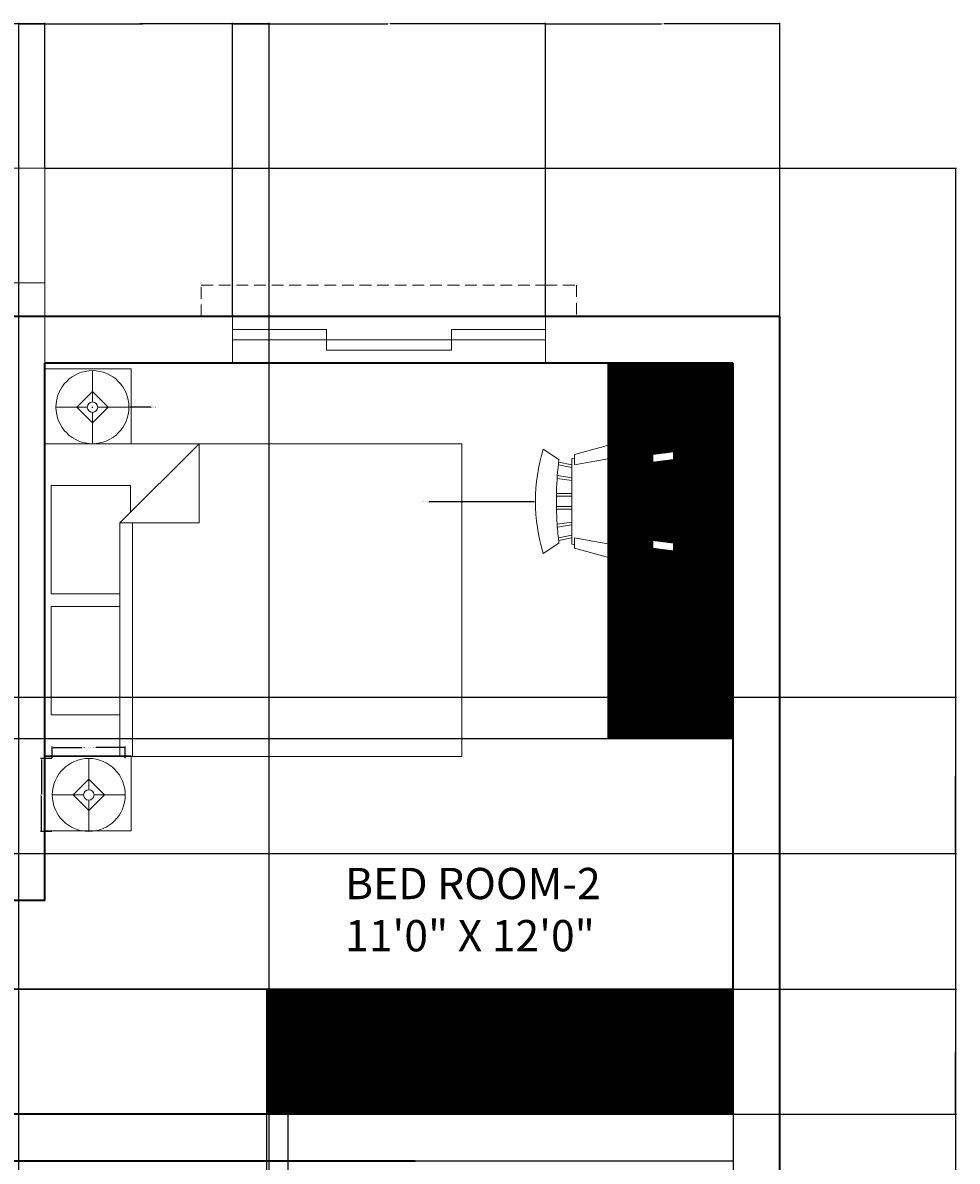
# Model space of a CAD drawing. Units: inches. Extents: x 6662 to 7211, y 5077 to 5683.
# Tile 9 of 9: x 7032 to 7211, y 5465 to 5683. Entities that reach past the tile are written whole.
import ezdxf

# ---------------------------------------------------------------- set-up
doc = ezdxf.new("R2010")
doc.units = ezdxf.units.IN
doc.header["$LTSCALE"] = 3
doc.header["$MEASUREMENT"] = 0
doc.linetypes.add('HIDDEN', pattern=[0.375, 0.25, -0.125])
for name, color, linetype, lineweight in [('A-ANNO-DIMS', 2, 'Continuous', 18), ('A-AREA-IDEN', 7, 'Continuous', 18), ('A-FLOR-CASE', 8, 'Continuous', 20), ('A-FLOR-CASE-PATT', 241, 'Continuous', 13), ('A-FLOR-PROJ', 7, 'Continuous', 18), ('A-FURN', 8, 'Continuous', 18), ('A-GLAZ', 4, 'Continuous', 18), ('A-GLAZ-OVHD', 4, 'HIDDEN', 13), ('A-WALL', 7, 'Continuous', 35)]:
    doc.layers.add(name, color=color, linetype=linetype, lineweight=lineweight)
doc.styles.get("Standard").update_dxf_attribs({"font": 'arial.ttf'})
doc.dimstyles.get("Standard").update_dxf_attribs({"dimtxt": 0.18, "dimasz": 0.18, "dimexe": 0.18, "dimexo": 0.0625, "dimgap": 0.09, "dimtad": 0, "dimtih": 1, "dimtoh": 1, "dimdec": 4, "dimzin": 0, "dimdsep": 46, "dimtxsty": 'Standard', "dimcen": 0.09, "dimadec": 0, "dimazin": 0, "dimtfac": 1, "dimtdec": 4, "dimtofl": 0, "dimtmove": 0, "dimatfit": 3, "dimfxl": 1, "dimtolj": 1, "dimtzin": 0, "dimarcsym": 0})

# ---------------------------------------------------------------- blocks, each defined once
blk = doc.blocks.new('Chair - Rocking')
for p, q in [((-8, -4.5), (-10, -1.5)), ((8, -4.5), (10, -1.5)), ((-4.5, -7), (-4.96674, -4.19951)), ((-4, -7), (-4.40532, -4.16272)), ((-1.5, -4.05012), (-1.5, -7)), ((-1, -7), (-1, -4.05012)), ((1, -7), (1, -4.04655)), ((1.5, -4.05012), (1.5, -7)), ((4, -7), (4.40187, -4.18694)), ((4.5, -7), (4.96761, -4.19437)), ((-7.5, -4.5), (-7, -7)), ((-6.5, -7), (-7.02225, -4.43)), ((6.5, -7), (7, -4.4057)), ((7.5, -4.5), (7, -7)), ((-9, -7.5), (-12, -18.49999)), ((-7, -7.5), (-9, -7.5)), ((-9, -18.49999), (-7, -7.5)), ((-8.23428, -6.99939), (-8.3093, -7.47958)), ((-8.23041, -7), (8.23915, -7)), ((7, -7.5), (9, -7.5)), ((9, -18.49999), (7, -7.5)), ((8.31071, -7.48854), (8.23449, -7.00073)), ((9, -7.5), (12, -18.49999)), ((-10.36644, -20.64523), (-10.5, -21.49999)), ((10.5, -21.49999), (10.3575, -20.58798)), ((-9, -22.49999), (-9.5, -26.49999)), ((0, -22.49999), (-9.5, -22.49999)), ((-8, -26.49999), (-7.5, -22.49999)), ((0, -22.49999), (9.5, -22.49999)), ((8, -26.49999), (7.5, -22.49999)), ((9, -22.49999), (9.5, -26.49999)), ((-9.5, -26.49999), (-8, -26.49999)), ((9.5, -26.49999), (8, -26.49999))]:
    blk.add_line(p, q)
for centre, radius, start, end in [((0, -34.08333), 34.08333, 72.93847, 107.0615), ((0, -68.25004), 64.25, 93.92211, 97.15267), ((0, -68.25004), 64.25, 82.84733, 93.92211), ((-10.5, -18.99999), 1.58114, 161.5651, 18.43495), ((10.5, -18.99999), 1.58114, 161.5651, 18.43495), ((-9.5, -21.49999), 1, 180, 270), ((9.5, -21.49999), 1, 270, 0)]:
    blk.add_arc(centre, radius, start, end)
blk = doc.blocks.new('Bed - Queen')
for p, q in [((0, -80.00003), (0, 0)), ((0, 0), (59.99999, 0)), ((59.99999, 0), (59.99999, -80.00003)), ((7.99999, -1.2), (28.79998, -1.2)), ((7.99999, -14.4), (7.99999, -1.2)), ((28.79998, -1.2), (28.79998, -14.4)), ((31.19999, -1.2), (51.99999, -1.2)), ((31.19999, -14.4), (31.19999, -1.2)), ((51.99999, -1.2), (51.99999, -16.4)), ((0, -14.4), (44.8, -14.4)), ((59.99999, -29.6), (44.8, -14.4)), ((44.8, -14.4), (44.8, -29.6)), ((44.8, -16.8), (0, -16.8)), ((51.99999, -16.4), (46.79936, -16.4)), ((44.8, -29.6), (59.99999, -29.6)), ((59.99999, -80.00003), (0, -80.00003))]:
    blk.add_line(p, q)
blk = doc.blocks.new('Lamp - Table')
for p, q in [((0, 7), (0, 1)), ((0, 3), (-3, 0)), ((3, 0), (0, 3)), ((-1, 0), (-7, 0)), ((-3, 0), (0, -3)), ((0, -3), (3, 0)), ((1, 0), (7, 0)), ((0, -1), (0, -7))]:
    blk.add_line(p, q)
for radius in [7, 1]:
    blk.add_circle((0, 0), radius)
blk = doc.blocks.new('BEDSIDE-TABLE')
blk.add_lwpolyline([(0, 14.35), (16.56, 14.35), (16.56, 0), (0, 0)], close=True)
blk = doc.blocks.new('*D16')
at = {"layer": 'A-ANNO-DIMS', "color": 0, "lineweight": -2, "ltscale": 3, "transparency": 16777216}
for p, q in [((7037.28, 5541.89), (7037.28, 5544.11)), ((7037.46, 5543.93), (7042.94, 5543.93)), ((7051.1, 5543.93), (7045.62, 5543.93)), ((7051.28, 5541.89), (7051.28, 5544.11))]:
    blk.add_line(p, q, dxfattribs=at)
at = {"layer": 'A-ANNO-DIMS', "color": 0, "ltscale": 3, "transparency": 16777216}
for points in [[(7037.46, 5543.96), (7037.46, 5543.9), (7037.28, 5543.93)], [(7051.1, 5543.96), (7051.1, 5543.9), (7051.28, 5543.93)]]:
    blk.add_solid(points, dxfattribs=at)
at = {"layer": 'Defpoints', "color": 0, "ltscale": 3, "transparency": 16777216}
for p in [(7051.28, 5543.93), (7037.28, 5541.83), (7051.28, 5541.83)]:
    blk.add_point(p, dxfattribs=at)
at = {"layer": 'A-ANNO-DIMS', "color": 0, "ltscale": 3, "transparency": 16777216, "insert": (7044.28, 5543.93), "char_height": 0.18, "attachment_point": 5}
blk.add_mtext('\\A1;TABLE LAMP 14 TYP.', dxfattribs=at)
blk = doc.blocks.new('*D17')
at = {"layer": 'A-ANNO-DIMS', "color": 0, "lineweight": -2, "ltscale": 3, "transparency": 16777216}
for p, q in [((7037.21, 5541.83), (7035, 5541.83)), ((7035.18, 5541.65), (7035.18, 5535.01)), ((7035.18, 5528.01), (7035.18, 5534.65)), ((7037.21, 5527.83), (7035, 5527.83))]:
    blk.add_line(p, q, dxfattribs=at)
at = {"layer": 'A-ANNO-DIMS', "color": 0, "ltscale": 3, "transparency": 16777216}
for points in [[(7035.15, 5541.65), (7035.21, 5541.65), (7035.18, 5541.83)], [(7035.15, 5528.01), (7035.21, 5528.01), (7035.18, 5527.83)]]:
    blk.add_solid(points, dxfattribs=at)
at = {"layer": 'Defpoints', "color": 0, "ltscale": 3, "transparency": 16777216}
for p in [(7035.18, 5541.83), (7037.28, 5541.83), (7037.28, 5527.83)]:
    blk.add_point(p, dxfattribs=at)
at = {"layer": 'A-ANNO-DIMS', "color": 0, "ltscale": 3, "transparency": 16777216, "insert": (7035.18, 5534.83), "char_height": 0.18, "attachment_point": 5}
blk.add_mtext('\\A1;14 TYP.', dxfattribs=at)
blk = doc.blocks.new('*D41')
at = {"layer": 'A-ANNO-DIMS', "color": 0, "lineweight": -2, "ltscale": 3, "transparency": 16777216}
for p, q in [((7035.92, 5655.02), (7210.74, 5655.02)), ((7210.56, 5654.84), (7210.56, 5379.99)), ((7210.56, 5104.78), (7210.56, 5379.63)), ((7010.92, 5104.6), (7210.74, 5104.6))]:
    blk.add_line(p, q, dxfattribs=at)
at = {"layer": 'A-ANNO-DIMS', "color": 0, "ltscale": 3, "transparency": 16777216}
for points in [[(7210.53, 5654.84), (7210.59, 5654.84), (7210.56, 5655.02)], [(7210.53, 5104.78), (7210.59, 5104.78), (7210.56, 5104.6)]]:
    blk.add_solid(points, dxfattribs=at)
at = {"layer": 'Defpoints', "color": 0, "ltscale": 3, "transparency": 16777216}
for p in [(7035.86, 5655.02), (7210.56, 5655.02), (7010.86, 5104.6)]:
    blk.add_point(p, dxfattribs=at)
at = {"layer": 'A-ANNO-DIMS', "color": 0, "ltscale": 3, "transparency": 16777216, "insert": (7210.56, 5379.81), "char_height": 0.18, "attachment_point": 5}
blk.add_mtext('\\A1;550.4', dxfattribs=at)
blk = doc.blocks.new('*D46')
at = {"layer": 'A-ANNO-DIMS', "color": 0, "lineweight": -2, "ltscale": 3, "transparency": 16777216}
for p, q in [((6869.86, 5655.08), (6869.86, 5682.9)), ((6870.04, 5682.72), (6952.58, 5682.72)), ((7035.68, 5682.72), (6953.14, 5682.72)), ((7035.86, 5655.08), (7035.86, 5682.9))]:
    blk.add_line(p, q, dxfattribs=at)
at = {"layer": 'A-ANNO-DIMS', "color": 0, "ltscale": 3, "transparency": 16777216}
for points in [[(6870.04, 5682.75), (6870.04, 5682.69), (6869.86, 5682.72)], [(7035.68, 5682.75), (7035.68, 5682.69), (7035.86, 5682.72)]]:
    blk.add_solid(points, dxfattribs=at)
at = {"layer": 'Defpoints', "color": 0, "ltscale": 3, "transparency": 16777216}
for p in [(7035.86, 5682.72), (6869.86, 5655.02), (7035.86, 5655.02)]:
    blk.add_point(p, dxfattribs=at)
at = {"layer": 'A-ANNO-DIMS', "color": 0, "ltscale": 3, "transparency": 16777216, "insert": (6952.86, 5682.72), "char_height": 0.18, "attachment_point": 5}
blk.add_mtext('\\A1;166', dxfattribs=at)
blk = doc.blocks.new('*D47')
at = {"layer": 'A-ANNO-DIMS', "color": 0, "lineweight": -2, "ltscale": 3, "transparency": 16777216}
for p, q in [((7035.86, 5655.08), (7035.86, 5682.9)), ((7036.04, 5682.72), (7053.64, 5682.72)), ((7071.68, 5682.72), (7054.08, 5682.72)), ((7071.86, 5626.66), (7071.86, 5682.9))]:
    blk.add_line(p, q, dxfattribs=at)
at = {"layer": 'A-ANNO-DIMS', "color": 0, "ltscale": 3, "transparency": 16777216}
for points in [[(7036.04, 5682.75), (7036.04, 5682.69), (7035.86, 5682.72)], [(7071.68, 5682.75), (7071.68, 5682.69), (7071.86, 5682.72)]]:
    blk.add_solid(points, dxfattribs=at)
at = {"layer": 'Defpoints', "color": 0, "ltscale": 3, "transparency": 16777216}
for p in [(7071.86, 5682.72), (7035.86, 5655.02), (7071.86, 5626.6)]:
    blk.add_point(p, dxfattribs=at)
at = {"layer": 'A-ANNO-DIMS', "color": 0, "ltscale": 3, "transparency": 16777216, "insert": (7053.86, 5682.72), "char_height": 0.18, "attachment_point": 5}
blk.add_mtext('\\A1;36', dxfattribs=at)
blk = doc.blocks.new('*D48')
at = {"layer": 'A-ANNO-DIMS', "color": 0, "lineweight": -2, "ltscale": 3, "transparency": 16777216}
for p, q in [((7071.86, 5626.66), (7071.86, 5682.9)), ((7072.04, 5682.72), (7101.64, 5682.72)), ((7131.68, 5682.72), (7102.08, 5682.72)), ((7131.86, 5626.66), (7131.86, 5682.9))]:
    blk.add_line(p, q, dxfattribs=at)
at = {"layer": 'A-ANNO-DIMS', "color": 0, "ltscale": 3, "transparency": 16777216}
for points in [[(7072.04, 5682.75), (7072.04, 5682.69), (7071.86, 5682.72)], [(7131.68, 5682.75), (7131.68, 5682.69), (7131.86, 5682.72)]]:
    blk.add_solid(points, dxfattribs=at)
at = {"layer": 'Defpoints', "color": 0, "ltscale": 3, "transparency": 16777216}
for p in [(7131.86, 5682.72), (7071.86, 5626.6), (7131.86, 5626.6)]:
    blk.add_point(p, dxfattribs=at)
at = {"layer": 'A-ANNO-DIMS', "color": 0, "ltscale": 3, "transparency": 16777216, "insert": (7101.86, 5682.72), "char_height": 0.18, "attachment_point": 5}
blk.add_mtext('\\A1;60', dxfattribs=at)
blk = doc.blocks.new('*D49')
at = {"layer": 'A-ANNO-DIMS', "color": 0, "lineweight": -2, "ltscale": 3, "transparency": 16777216}
for p, q in [((7131.86, 5626.66), (7131.86, 5682.9)), ((7132.04, 5682.72), (7154.13, 5682.72)), ((7176.68, 5682.72), (7154.58, 5682.72)), ((7176.86, 5626.66), (7176.86, 5682.9))]:
    blk.add_line(p, q, dxfattribs=at)
at = {"layer": 'A-ANNO-DIMS', "color": 0, "ltscale": 3, "transparency": 16777216}
for points in [[(7132.04, 5682.75), (7132.04, 5682.69), (7131.86, 5682.72)], [(7176.68, 5682.75), (7176.68, 5682.69), (7176.86, 5682.72)]]:
    blk.add_solid(points, dxfattribs=at)
at = {"layer": 'Defpoints', "color": 0, "ltscale": 3, "transparency": 16777216}
for p in [(7176.86, 5682.72), (7131.86, 5626.6), (7176.86, 5626.6)]:
    blk.add_point(p, dxfattribs=at)
at = {"layer": 'A-ANNO-DIMS', "color": 0, "ltscale": 3, "transparency": 16777216, "insert": (7154.36, 5682.72), "char_height": 0.18, "attachment_point": 5}
blk.add_mtext('\\A1;45', dxfattribs=at)
blk = doc.blocks.new('*D68')
at = {"layer": 'A-ANNO-DIMS', "color": 0, "lineweight": -2, "ltscale": 3, "transparency": 16777216}
for p, q in [((6878.92, 5553.6), (7210.74, 5553.6)), ((7210.56, 5553.42), (7210.56, 5538.78)), ((7210.56, 5523.78), (7210.56, 5538.42)), ((6878.92, 5523.6), (7210.74, 5523.6))]:
    blk.add_line(p, q, dxfattribs=at)
at = {"layer": 'A-ANNO-DIMS', "color": 0, "ltscale": 3, "transparency": 16777216}
for points in [[(7210.53, 5553.42), (7210.59, 5553.42), (7210.56, 5553.6)], [(7210.53, 5523.78), (7210.59, 5523.78), (7210.56, 5523.6)]]:
    blk.add_solid(points, dxfattribs=at)
at = {"layer": 'Defpoints', "color": 0, "ltscale": 3, "transparency": 16777216}
for p in [(6878.86, 5553.6), (7210.56, 5553.6), (6878.86, 5523.6)]:
    blk.add_point(p, dxfattribs=at)
at = {"layer": 'A-ANNO-DIMS', "color": 0, "ltscale": 3, "transparency": 16777216, "insert": (7210.56, 5538.6), "char_height": 0.18, "attachment_point": 5}
blk.add_mtext('\\A1;30', dxfattribs=at)
blk = doc.blocks.new('*D75')
at = {"layer": 'A-ANNO-DIMS', "color": 0, "lineweight": -2, "ltscale": 3, "transparency": 16777216}
for p, q in [((7030.86, 5179.16), (7030.86, 5682.9)), ((7031.04, 5682.72), (7054.64, 5682.72)), ((7078.68, 5682.72), (7055.08, 5682.72)), ((7078.86, 5179.16), (7078.86, 5682.9))]:
    blk.add_line(p, q, dxfattribs=at)
at = {"layer": 'A-ANNO-DIMS', "color": 0, "ltscale": 3, "transparency": 16777216}
for points in [[(7031.04, 5682.75), (7031.04, 5682.69), (7030.86, 5682.72)], [(7078.68, 5682.75), (7078.68, 5682.69), (7078.86, 5682.72)]]:
    blk.add_solid(points, dxfattribs=at)
at = {"layer": 'Defpoints', "color": 0, "ltscale": 3, "transparency": 16777216}
for p in [(7078.86, 5682.72), (7030.86, 5179.1), (7078.86, 5179.1)]:
    blk.add_point(p, dxfattribs=at)
at = {"layer": 'A-ANNO-DIMS', "color": 0, "ltscale": 3, "transparency": 16777216, "insert": (7054.86, 5682.72), "char_height": 0.18, "attachment_point": 5}
blk.add_mtext('\\A1;48', dxfattribs=at)
blk = doc.blocks.new('*D76')
at = {"layer": 'A-ANNO-DIMS', "color": 0, "lineweight": -2, "ltscale": 3, "transparency": 16777216}
for p, q in [((7167.8, 5464.6), (6661.98, 5464.6)), ((6662.16, 5464.42), (6662.16, 5449.65)), ((6662.16, 5434.53), (6662.16, 5449.29)), ((7167.8, 5434.35), (6661.98, 5434.35))]:
    blk.add_line(p, q, dxfattribs=at)
at = {"layer": 'A-ANNO-DIMS', "color": 0, "ltscale": 3, "transparency": 16777216}
for points in [[(6662.13, 5464.42), (6662.19, 5464.42), (6662.16, 5464.6)], [(6662.13, 5434.53), (6662.19, 5434.53), (6662.16, 5434.35)]]:
    blk.add_solid(points, dxfattribs=at)
at = {"layer": 'Defpoints', "color": 0, "ltscale": 3, "transparency": 16777216}
for p in [(7167.86, 5464.6), (6662.16, 5434.35), (7167.86, 5434.35)]:
    blk.add_point(p, dxfattribs=at)
at = {"layer": 'A-ANNO-DIMS', "color": 0, "ltscale": 3, "transparency": 16777216, "insert": (6662.16, 5449.47), "char_height": 0.18, "attachment_point": 5}
blk.add_mtext('\\A1;30.25', dxfattribs=at)
blk = doc.blocks.new('*D80')
at = {"layer": 'A-ANNO-DIMS', "color": 0, "lineweight": -2, "ltscale": 3, "transparency": 16777216}
for p, q in [((6825.96, 5497.6), (7210.74, 5497.6)), ((7210.56, 5497.42), (7210.56, 5485.78)), ((7210.56, 5473.78), (7210.56, 5485.42)), ((6825.96, 5473.6), (7210.74, 5473.6))]:
    blk.add_line(p, q, dxfattribs=at)
at = {"layer": 'A-ANNO-DIMS', "color": 0, "ltscale": 3, "transparency": 16777216}
for points in [[(7210.53, 5497.42), (7210.59, 5497.42), (7210.56, 5497.6)], [(7210.53, 5473.78), (7210.59, 5473.78), (7210.56, 5473.6)]]:
    blk.add_solid(points, dxfattribs=at)
at = {"layer": 'Defpoints', "color": 0, "ltscale": 3, "transparency": 16777216}
for p in [(6825.9, 5497.6), (7210.56, 5497.6), (6825.9, 5473.6)]:
    blk.add_point(p, dxfattribs=at)
at = {"layer": 'A-ANNO-DIMS', "color": 0, "ltscale": 3, "transparency": 16777216, "insert": (7210.56, 5485.6), "char_height": 0.18, "attachment_point": 5}
blk.add_mtext('\\A1;24', dxfattribs=at)
blk = doc.blocks.new('*D81')
at = {"layer": 'A-ANNO-DIMS', "color": 0, "lineweight": -2, "ltscale": 3, "transparency": 16777216}
for p, q in [((7078.36, 5473.54), (7078.36, 5076.72)), ((7167.86, 5473.54), (7167.86, 5076.72)), ((7078.54, 5076.9), (7122.78, 5076.9)), ((7167.68, 5076.9), (7123.43, 5076.9))]:
    blk.add_line(p, q, dxfattribs=at)
at = {"layer": 'A-ANNO-DIMS', "color": 0, "ltscale": 3, "transparency": 16777216}
for points in [[(7078.54, 5076.93), (7078.54, 5076.87), (7078.36, 5076.9)], [(7167.68, 5076.93), (7167.68, 5076.87), (7167.86, 5076.9)]]:
    blk.add_solid(points, dxfattribs=at)
at = {"layer": 'Defpoints', "color": 0, "ltscale": 3, "transparency": 16777216}
for p in [(7078.36, 5473.6), (7167.86, 5473.6), (7167.86, 5076.9)]:
    blk.add_point(p, dxfattribs=at)
at = {"layer": 'A-ANNO-DIMS', "color": 0, "ltscale": 3, "transparency": 16777216, "insert": (7123.11, 5076.9), "char_height": 0.18, "attachment_point": 5}
blk.add_mtext('\\A1;89.5', dxfattribs=at)
blk = doc.blocks.new('*D82')
at = {"layer": 'A-ANNO-DIMS', "color": 0, "lineweight": -2, "ltscale": 3, "transparency": 16777216}
for p, q in [((7167.8, 5545.6), (6661.98, 5545.6)), ((6662.16, 5545.42), (6662.16, 5521.78)), ((6662.16, 5497.78), (6662.16, 5521.42)), ((7167.8, 5497.6), (6661.98, 5497.6))]:
    blk.add_line(p, q, dxfattribs=at)
at = {"layer": 'A-ANNO-DIMS', "color": 0, "ltscale": 3, "transparency": 16777216}
for points in [[(6662.13, 5545.42), (6662.19, 5545.42), (6662.16, 5545.6)], [(6662.13, 5497.78), (6662.19, 5497.78), (6662.16, 5497.6)]]:
    blk.add_solid(points, dxfattribs=at)
at = {"layer": 'Defpoints', "color": 0, "ltscale": 3, "transparency": 16777216}
for p in [(6662.16, 5545.6), (7167.86, 5545.6), (7167.86, 5497.6)]:
    blk.add_point(p, dxfattribs=at)
at = {"layer": 'A-ANNO-DIMS', "color": 0, "ltscale": 3, "transparency": 16777216, "insert": (6662.16, 5521.6), "char_height": 0.18, "attachment_point": 5}
blk.add_mtext('\\A1;48', dxfattribs=at)
blk = doc.blocks.new('*D103')
at = {"layer": 'A-ANNO-DIMS', "color": 0, "lineweight": -2, "ltscale": 3, "transparency": 16777216}
for p, q in [((7082.65, 5477.61), (7082.47, 5477.61)), ((7082.47, 5477.61), (7082.47, 5441.64)), ((7082.38, 5381.21), (7082.56, 5381.21)), ((7082.47, 5381.12), (7082.47, 5381.3))]:
    blk.add_line(p, q, dxfattribs=at)
at = {"layer": 'A-ANNO-DIMS', "color": 0, "ltscale": 3, "transparency": 16777216}
blk.add_solid([(7082.44, 5441.64), (7082.5, 5441.64), (7082.47, 5441.46)], dxfattribs=at)
at = {"layer": 'Defpoints', "color": 0, "ltscale": 3, "transparency": 16777216}
for p in [(7082.47, 5441.46), (7082.47, 5381.21)]:
    blk.add_point(p, dxfattribs=at)
at = {"layer": 'A-ANNO-DIMS', "color": 0, "ltscale": 3, "transparency": 16777216, "insert": (7083.32, 5477.61), "char_height": 0.18, "attachment_point": 5}
blk.add_mtext('\\A1;2X R60.25', dxfattribs=at)
blk = doc.blocks.new('*D105')
at = {"layer": 'A-ANNO-DIMS', "color": 0, "lineweight": -2, "ltscale": 3, "transparency": 16777216}
for p, q in [((7109.51, 5591.13), (7129.78, 5591.13)), ((7163.96, 5591.13), (7164.14, 5591.13)), ((7164.05, 5591.04), (7164.05, 5591.22))]:
    blk.add_line(p, q, dxfattribs=at)
at = {"layer": 'A-ANNO-DIMS', "color": 0, "ltscale": 3, "transparency": 16777216}
blk.add_solid([(7129.78, 5591.16), (7129.78, 5591.1), (7129.96, 5591.13)], dxfattribs=at)
at = {"layer": 'Defpoints', "color": 0, "ltscale": 3, "transparency": 16777216}
for p in [(7129.96, 5591.13), (7164.05, 5591.13)]:
    blk.add_point(p, dxfattribs=at)
at = {"layer": 'A-ANNO-DIMS', "color": 0, "ltscale": 3, "transparency": 16777216, "insert": (7108.84, 5591.13), "char_height": 0.18, "attachment_point": 5}
blk.add_mtext('\\A1;3X R34.08', dxfattribs=at)
blk = doc.blocks.new('*D106')
at = {"layer": 'A-ANNO-DIMS', "color": 0, "lineweight": -2, "ltscale": 3, "transparency": 16777216}
for p, q in [((7044.89, 5609.19), (7045.07, 5609.19)), ((7044.98, 5609.1), (7044.98, 5609.28)), ((7056.18, 5609.19), (7052.16, 5609.19))]:
    blk.add_line(p, q, dxfattribs=at)
at = {"layer": 'A-ANNO-DIMS', "color": 0, "ltscale": 3, "transparency": 16777216}
blk.add_solid([(7052.16, 5609.22), (7052.16, 5609.16), (7051.98, 5609.19)], dxfattribs=at)
at = {"layer": 'Defpoints', "color": 0, "ltscale": 3, "transparency": 16777216}
for p in [(7037.98, 5609.19), (7051.98, 5609.19)]:
    blk.add_point(p, dxfattribs=at)
at = {"layer": 'A-ANNO-DIMS', "color": 0, "ltscale": 3, "transparency": 16777216, "insert": (7056.69, 5609.19), "char_height": 0.18, "attachment_point": 5}
blk.add_mtext('\\A1;6X ∅14', dxfattribs=at)

msp = doc.modelspace()

# ---------------------------------------------------------------- hatches: boundary and pattern name
at = {"layer": 'A-FLOR-CASE-PATT'}
h = msp.add_hatch(dxfattribs=at)
h.set_pattern_fill('ANSI31', color=256)
h.paths.add_polyline_path([(7167.8579, 5617.5979), (7143.8579, 5617.5979), (7143.8579, 5545.5979), (7167.8579, 5545.5979)])
h.paths.add_polyline_path([(7152.4639, 5591.1311), (7152.4639, 5600.1311), (7156.4639, 5600.6311), (7156.4639, 5599.1311), (7152.4639, 5598.6311), (7152.4639, 5591.1311), (7152.4639, 5583.6311), (7156.4639, 5583.1311), (7156.4639, 5581.6311), (7152.4639, 5582.1311)], flags=16)
h = msp.add_hatch(dxfattribs=at)
h.set_pattern_fill('ANSI31', color=256)
h.paths.add_polyline_path([(6869.8579, 5283.7981), (6845.8579, 5283.7981), (6845.8579, 5229.4653), (6847.018, 5229.7817, -0.54116316), (6849.0925, 5228.1371), (6849.7129, 5228.234, -0.50821327), (6851.018, 5227.2817), (6851.018, 5226.7817), (6855.018, 5227.2817), (6855.018, 5225.7817), (6851.018, 5225.2817), (6851.018, 5217.7817), (6851.018, 5210.2817), (6855.018, 5209.7817), (6855.018, 5208.2817), (6851.018, 5208.7817), (6851.018, 5208.2817, -0.41421356), (6850.018, 5207.2817), (6849.0925, 5207.4263, -0.50580924), (6847.1872, 5205.7355), (6845.8579, 5206.0981), (6845.8579, 5179.0979), (6869.8579, 5179.0979)])
h.paths.add_polyline_path([(7167.8579, 5497.5979), (7143.8579, 5497.5979), (7078.3579, 5497.5979), (7078.3579, 5473.5979), (7163.8579, 5473.5979), (7167.8579, 5473.5979)])
h.paths.add_polyline_path([(6825.9016, 5497.5979), (6725.8579, 5497.5979), (6725.8579, 5473.5979), (6825.9016, 5473.5979)])
h.paths.add_polyline_path([(6796.6359, 5485.2095), (6797.1359, 5489.2095), (6806.1359, 5489.2095), (6815.1359, 5489.2095), (6815.6359, 5485.2095), (6814.1359, 5485.2095), (6813.6359, 5489.2095), (6806.1359, 5489.2095), (6798.6359, 5489.2095), (6798.1359, 5485.2095)], flags=16)

# ---------------------------------------------------------------- linework, layer by layer
at = {"layer": 'A-FLOR-CASE'}
for p, q in [((7143.8579, 5545.5979), (7143.8579, 5617.5979)), ((7167.8579, 5545.5979), (7143.8579, 5545.5979)), ((7143.8579, 5497.5979), (7078.3579, 5497.5979)), ((7078.3579, 5473.5979), (7078.3579, 5497.5979)), ((7143.8579, 5497.5979), (7167.8579, 5497.5979))]:
    msp.add_line(p, q, dxfattribs=at)
at = {"layer": 'A-FLOR-PROJ', "ltscale": 3}
for p, q in [((7035.8579, 5655.0209), (6950.8579, 5655.0209)), ((7035.8579, 5617.5979), (7035.8579, 5655.0209)), ((7026.8579, 5633.0136), (7035.8579, 5633.0136))]:
    msp.add_line(p, q, dxfattribs=at)
at = {"layer": 'A-GLAZ'}
for p, q in [((7071.8579, 5617.5979), (7071.8579, 5626.5979)), ((7131.8579, 5617.5979), (7131.8579, 5626.5979)), ((7089.8579, 5624.0979), (7071.8579, 5624.0979)), ((7089.8579, 5620.0979), (7089.8579, 5624.0979)), ((7113.8579, 5620.0979), (7113.8579, 5624.0979)), ((7131.8579, 5624.0979), (7113.8579, 5624.0979)), ((7131.8579, 5622.0979), (7071.8579, 5622.0979)), ((7113.8579, 5620.0979), (7089.8579, 5620.0979))]:
    msp.add_line(p, q, dxfattribs=at)
at = {"layer": 'A-GLAZ-OVHD', "ltscale": 3}
for p, q in [((7065.8579, 5626.5979), (7065.8579, 5632.5979)), ((7065.8579, 5632.5979), (7131.8579, 5632.5979)), ((7131.8579, 5632.5979), (7137.8579, 5632.5979)), ((7137.8579, 5632.5979), (7137.8579, 5626.5979)), ((7071.8579, 5626.5979), (7065.8579, 5626.5979))]:
    msp.add_line(p, q, dxfattribs=at)
at = {"layer": 'A-WALL'}
for p, q in [((7176.8579, 5626.5979), (6716.8579, 5626.5979)), ((7176.8579, 5434.3479), (7176.8579, 5626.5979)), ((7035.8579, 5514.5979), (7035.8579, 5617.5979)), ((7167.8579, 5617.5979), (7035.8579, 5617.5979)), ((7167.8579, 5617.5979), (7107.8579, 5617.5979)), ((7167.8579, 5473.5979), (7167.8579, 5617.5979)), ((7167.8579, 5473.5979), (7167.8579, 5617.5979)), ((7035.8579, 5514.5979), (7024.8579, 5514.5979)), ((7163.8579, 5473.5979), (6992.8579, 5473.5979)), ((7167.8579, 5473.5979), (7031.8579, 5473.5979)), ((7106.8579, 5464.5979), (6992.8579, 5464.5979))]:
    msp.add_line(p, q, dxfattribs=at)

# ---------------------------------------------------------------- block references
at = {"layer": 'A-FURN'}
for name, p in [('BEDSIDE-TABLE', (7035.858, 5602.1913)), ('Lamp - Table', (7044.98, 5609.1914)), ('BEDSIDE-TABLE', (7035.858, 5527.9576)), ('Lamp - Table', (7044.2766, 5534.8292))]:
    msp.add_blockref(name, p, dxfattribs=at)
at = {"layer": 'A-FURN', "rotation": 90}
for name, p in [('Bed - Queen', (7035.8579, 5542.191)), ('Chair - Rocking', (7129.9639, 5591.1311))]:
    msp.add_blockref(name, p, dxfattribs=at)

# ---------------------------------------------------------------- texts
at = {"layer": 'A-AREA-IDEN', "ltscale": 3, "insert": (7093.4345, 5520.8483), "char_height": 6, "attachment_point": 1}
msp.add_mtext_dynamic_manual_height_columns('BED ROOM-2\\P11\'0" X 12\'0"', width=381.547883, gutter_width=1, heights=[0], dxfattribs=at)

# ---------------------------------------------------------------- dimensions: what is measured, and where the dimension line sits
at = {"layer": 'A-ANNO-DIMS', "ltscale": 3}
for base, p1, p2, override, picture, middle in [((7035.8579, 5682.7209), (6869.8579, 5655.0209), (7035.8579, 5655.0209), {"dimdec": 0, "dimlfac": 1, "dimrnd": 0, "dimzin": 0, "dimdsep": 46, "dimlunit": 2}, '*D46', (6952.8579, 5682.7209)), ((7078.8579, 5682.7209), (7030.8579, 5179.0979), (7078.8579, 5179.0979), {"dimdec": 0, "dimlfac": 1, "dimrnd": 0, "dimzin": 0, "dimdsep": 46, "dimlunit": 2}, '*D75', (7054.8579, 5682.7209)), ((7071.8579, 5682.7209), (7035.8579, 5655.0209), (7071.8579, 5626.5979), {"dimdec": 0, "dimlfac": 1, "dimrnd": 0, "dimzin": 0, "dimdsep": 46, "dimlunit": 2}, '*D47', (7053.8579, 5682.7209)), ((7131.8579, 5682.7209), (7071.8579, 5626.5979), (7131.8579, 5626.5979), {"dimdec": 0, "dimlfac": 1, "dimrnd": 0, "dimzin": 0, "dimdsep": 46, "dimlunit": 2}, '*D48', (7101.8579, 5682.7209)), ((7176.8579, 5682.7209), (7131.8579, 5626.5979), (7176.8579, 5626.5979), {"dimdec": 0, "dimlfac": 1, "dimrnd": 0, "dimzin": 0, "dimdsep": 46, "dimlunit": 2}, '*D49', (7154.3579, 5682.7209)), ((7167.8579, 5076.8979), (7078.3579, 5473.5979), (7167.8579, 5473.5979), {"dimdec": 1, "dimlfac": 1, "dimrnd": 0, "dimzin": 0, "dimdsep": 46, "dimlunit": 2}, '*D81', (7123.1079, 5076.8979))]:
    dim = msp.add_linear_dim(base=base, p1=p1, p2=p2, dimstyle='Standard', override=override, dxfattribs=at)
    dim.commit()
    dim.dimension.update_dxf_attribs({"geometry": picture, "text_midpoint": middle})
for base, p1, p2, override, picture, middle in [((7210.5579, 5655.0209), (7010.8579, 5104.5979), (7035.8579, 5655.0209), {"dimdec": 1, "dimlfac": 1, "dimrnd": 0, "dimzin": 0, "dimdsep": 46, "dimlunit": 2}, '*D41', (7210.5579, 5379.8094)), ((7210.5579, 5553.5979), (6878.8579, 5523.5979), (6878.8579, 5553.5979), {"dimdec": 0, "dimlfac": 1, "dimrnd": 0, "dimzin": 0, "dimdsep": 46, "dimlunit": 2}, '*D68', (7210.5579, 5538.5979)), ((6662.1579, 5545.5979), (7167.8579, 5497.5979), (7167.8579, 5545.5979), {"dimdec": 0, "dimlfac": 1, "dimrnd": 0, "dimzin": 0, "dimdsep": 46, "dimlunit": 2}, '*D82', (6662.1579, 5521.5979)), ((7210.5579, 5497.5979), (6825.9016, 5473.5979), (6825.9016, 5497.5979), {"dimdec": 0, "dimlfac": 1, "dimrnd": 0, "dimzin": 0, "dimdsep": 46, "dimlunit": 2}, '*D80', (7210.5579, 5485.5979)), ((6662.1579, 5434.3479), (7167.8579, 5464.5979), (7167.8579, 5434.3479), {"dimdec": 2, "dimlfac": 1, "dimrnd": 0, "dimzin": 0, "dimdsep": 46, "dimlunit": 2}, '*D76', (6662.1579, 5449.4729))]:
    dim = msp.add_linear_dim(base=base, p1=p1, p2=p2, angle=90, dimstyle='Standard', override=override, dxfattribs=at)
    dim.commit()
    dim.dimension.update_dxf_attribs({"geometry": picture, "text_midpoint": middle})
dim = msp.add_diameter_dim_2p(p1=(7037.98, 5609.1919), p2=(7051.98, 5609.191), text='6X <>', dimstyle='Standard', override={"dimdec": 0, "dimlfac": 1, "dimrnd": 0, "dimzin": 0, "dimdsep": 46, "dimlunit": 2}, dxfattribs=at)
dim.commit()
dim.dimension.update_dxf_attribs({"geometry": '*D106', "text_midpoint": (7056.18, 5609.1907), "dimtype": 163})
for center, mpoint, text, picture, middle in [((7164.0473, 5591.1311), (7129.9639, 5591.131), '3X <>', '*D105', (7109.514, 5591.1309)), ((7082.466, 5381.2135), (7082.466, 5441.4635), '2X <>', '*D103', (7083.3214, 5477.6135))]:
    dim = msp.add_radius_dim(center=center, mpoint=mpoint, text=text, dimstyle='Standard', override={"dimdec": 2, "dimlfac": 1, "dimrnd": 0, "dimzin": 0, "dimdsep": 46, "dimlunit": 2}, dxfattribs=at)
    dim.commit()
    dim.dimension.update_dxf_attribs({"geometry": picture, "text_midpoint": middle, "dimtype": 164})
dim = msp.add_linear_dim(base=(7051.2766, 5543.9292), p1=(7037.2766, 5541.8292), p2=(7051.2766, 5541.8292), text='TABLE LAMP <> TYP.', dimstyle='Standard', override={"dimdec": 0, "dimlfac": 1, "dimrnd": 0, "dimzin": 0, "dimdsep": 46, "dimlunit": 2}, dxfattribs=at)
dim.commit()
dim.dimension.update_dxf_attribs({"geometry": '*D16', "text_midpoint": (7044.2766, 5543.9292)})
dim = msp.add_linear_dim(base=(7035.1766, 5541.8292), p1=(7037.2766, 5527.8292), p2=(7037.2766, 5541.8292), angle=90, text='<> TYP.', dimstyle='Standard', override={"dimdec": 0, "dimlfac": 1, "dimrnd": 0, "dimzin": 0, "dimdsep": 46, "dimlunit": 2}, dxfattribs=at)
dim.commit()
dim.dimension.update_dxf_attribs({"geometry": '*D17', "text_midpoint": (7035.1766, 5534.8292)})

doc.saveas('drawing.dxf')
